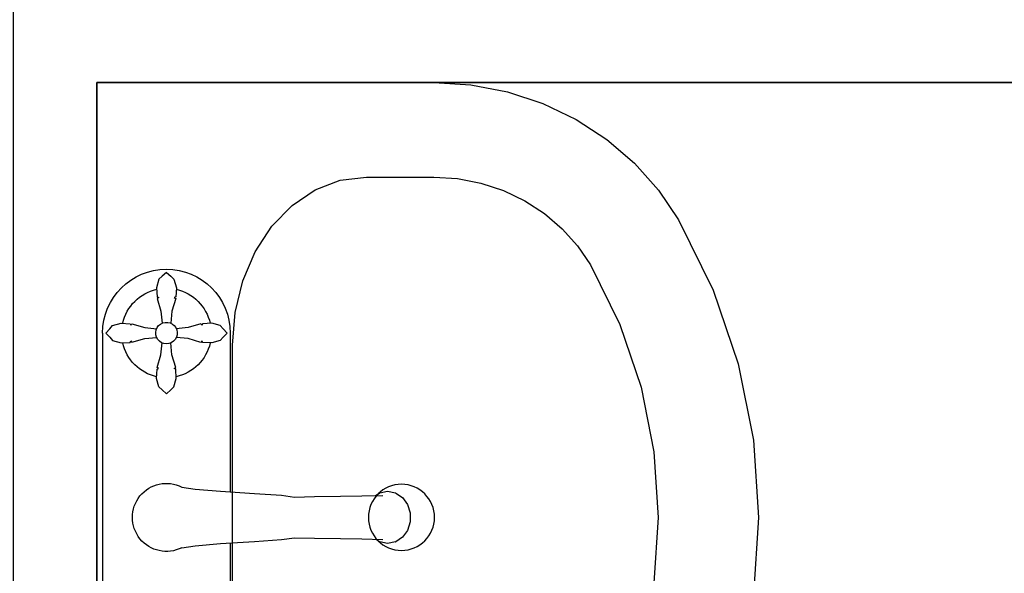
# Model space of a CAD drawing. Units: inches. Extents: x 3321 to 5237, y 11 to 1752.
# Tile 31 of 43: x 5059.68 to 5077.55, y 1416.43 to 1426.48. Entities that reach past the tile are written whole.
import ezdxf

# ---------------------------------------------------------------- set-up
doc = ezdxf.new("R2010")
doc.units = ezdxf.units.IN
for name, color, linetype, lineweight in [('A-ANNO-DIMS', 2, 'Continuous', 18), ('A-WALL', 7, 'Continuous', 35), ('Сантехника', 7, 'Continuous', 18)]:
    doc.layers.add(name, color=color, linetype=linetype, lineweight=lineweight)
doc.layers.add('SANTEH', color=7, linetype='Continuous')
doc.styles.get("Standard").update_dxf_attribs({"font": 'arial.ttf'})
doc.dimstyles.new('ISO-25', dxfattribs={"dimtxt": 9, "dimasz": 2.5, "dimexe": 1.25, "dimexo": 0.625, "dimtad": 1, "dimdec": 1, "dimlunit": 3, "dimtxsty": 'Standard', "dimcen": 2.5, "dimclrd": 4, "dimclre": 4, "dimclrt": 256, "dimadec": 0, "dimazin": 0, "dimtfac": 1, "dimtdec": 1, "dimtmove": 0, "dimatfit": 3, "dimfxl": 1, "dimarcsym": 0})

# ---------------------------------------------------------------- blocks, each defined once
blk = doc.blocks.new('Basin 01_71')
at = {"layer": 'SANTEH'}
for p, q in [((0.01, 350), (0.01, 171.82)), ((459.99, 350), (0.01, 350)), ((459.99, 350), (459.99, 171.82)), ((132.5, 345.3), (130.25, 343.2)), ((132.5, 345.3), (130.25, 343.2)), ((132.5, 345.3), (130.25, 343.2)), ((132.5, 345.3), (130.25, 343.2)), ((132.5, 345.3), (130.25, 343.2)), ((132.5, 345.3), (130.25, 343.2)), ((132.5, 346.95), (327.5, 346.95)), ((132.5, 345.3), (134.73, 343.2)), ((132.5, 345.3), (134.73, 343.2)), ((132.5, 345.3), (134.73, 343.2)), ((132.5, 345.3), (134.73, 343.2)), ((132.5, 345.3), (134.73, 343.2)), ((132.5, 345.3), (134.73, 343.2)), ((327.5, 345.3), (325.25, 343.2)), ((327.5, 345.3), (325.25, 343.2)), ((327.5, 345.3), (325.25, 343.2)), ((327.5, 345.3), (325.25, 343.2)), ((327.5, 345.3), (325.25, 343.2)), ((327.5, 345.3), (325.25, 343.2)), ((327.5, 345.3), (329.73, 343.2)), ((327.5, 345.3), (329.73, 343.2)), ((327.5, 345.3), (329.73, 343.2)), ((327.5, 345.3), (329.73, 343.2)), ((327.5, 345.3), (329.73, 343.2)), ((327.5, 345.3), (329.73, 343.2)), ((128.53, 341.7), (127.25, 337.2)), ((128.53, 341.7), (127.25, 337.2)), ((128.53, 341.7), (127.25, 337.2)), ((128.53, 341.7), (127.25, 337.2)), ((128.53, 341.7), (127.25, 337.2)), ((128.53, 341.7), (127.25, 337.2)), ((130.25, 343.2), (128.53, 341.7)), ((130.25, 343.2), (128.53, 341.7)), ((130.25, 343.2), (128.53, 341.7)), ((130.25, 343.2), (128.53, 341.7)), ((130.25, 343.2), (128.53, 341.7)), ((130.25, 343.2), (128.53, 341.7)), ((134.73, 343.2), (136.45, 341.7)), ((134.73, 343.2), (136.45, 341.7)), ((134.73, 343.2), (136.45, 341.7)), ((134.73, 343.2), (136.45, 341.7)), ((134.73, 343.2), (136.45, 341.7)), ((134.73, 343.2), (136.45, 341.7)), ((136.45, 341.7), (137.71, 337.2)), ((136.45, 341.7), (137.71, 337.2)), ((136.45, 341.7), (137.71, 337.2)), ((136.45, 341.7), (137.71, 337.2)), ((136.45, 341.7), (137.71, 337.2)), ((136.45, 341.7), (137.71, 337.2)), ((323.53, 341.7), (322.25, 337.2)), ((323.53, 341.7), (322.25, 337.2)), ((323.53, 341.7), (322.25, 337.2)), ((323.53, 341.7), (322.25, 337.2)), ((323.53, 341.7), (322.25, 337.2)), ((323.53, 341.7), (322.25, 337.2)), ((325.25, 343.2), (323.53, 341.7)), ((325.25, 343.2), (323.53, 341.7)), ((325.25, 343.2), (323.53, 341.7)), ((325.25, 343.2), (323.53, 341.7)), ((325.25, 343.2), (323.53, 341.7)), ((325.25, 343.2), (323.53, 341.7)), ((329.73, 343.2), (331.45, 341.7)), ((329.73, 343.2), (331.45, 341.7)), ((329.73, 343.2), (331.45, 341.7)), ((329.73, 343.2), (331.45, 341.7)), ((329.73, 343.2), (331.45, 341.7)), ((329.73, 343.2), (331.45, 341.7)), ((331.45, 341.7), (332.71, 337.2)), ((331.45, 341.7), (332.71, 337.2)), ((331.45, 341.7), (332.71, 337.2)), ((331.45, 341.7), (332.71, 337.2)), ((331.45, 341.7), (332.71, 337.2)), ((331.45, 341.7), (332.71, 337.2)), ((127.25, 337.2), (127.55, 332.32)), ((127.25, 337.2), (127.55, 332.32)), ((127.25, 337.2), (127.55, 332.32)), ((127.25, 337.2), (127.55, 332.32)), ((127.25, 337.2), (127.55, 332.32)), ((127.25, 337.2), (127.55, 332.32)), ((137.71, 337.2), (137.42, 332.32)), ((137.71, 337.2), (137.42, 332.32)), ((137.71, 337.2), (137.42, 332.32)), ((137.71, 337.2), (137.42, 332.32)), ((137.71, 337.2), (137.42, 332.32)), ((137.71, 337.2), (137.42, 332.32)), ((322.25, 337.2), (322.55, 332.32)), ((322.25, 337.2), (322.55, 332.32)), ((322.25, 337.2), (322.55, 332.32)), ((322.25, 337.2), (322.55, 332.32)), ((322.25, 337.2), (322.55, 332.32)), ((322.25, 337.2), (322.55, 332.32)), ((332.71, 337.2), (332.42, 332.32)), ((332.71, 337.2), (332.42, 332.32)), ((332.71, 337.2), (332.42, 332.32)), ((332.71, 337.2), (332.42, 332.32)), ((332.71, 337.2), (332.42, 332.32)), ((332.71, 337.2), (332.42, 332.32)), ((127.55, 332.32), (128.38, 332.02)), ((127.55, 332.32), (128.38, 332.02)), ((127.55, 332.32), (128.38, 332.02)), ((127.55, 332.32), (128.38, 332.02)), ((127.55, 332.32), (128.38, 332.02)), ((127.55, 332.32), (128.38, 332.02)), ((128.38, 332.02), (127.57, 331.46)), ((128.38, 332.02), (127.57, 331.46)), ((128.38, 332.02), (127.57, 331.46)), ((128.38, 332.02), (127.57, 331.46)), ((128.38, 332.02), (127.57, 331.46)), ((128.38, 332.02), (127.57, 331.46)), ((127.57, 331.46), (129.57, 324.71)), ((127.57, 331.46), (129.57, 324.71)), ((127.57, 331.46), (129.57, 324.71)), ((127.57, 331.46), (129.57, 324.71)), ((127.57, 331.46), (129.57, 324.71)), ((127.57, 331.46), (129.57, 324.71)), ((137.39, 331.46), (135.41, 324.71)), ((137.39, 331.46), (135.41, 324.71)), ((137.39, 331.46), (135.41, 324.71)), ((137.39, 331.46), (135.41, 324.71)), ((137.39, 331.46), (135.41, 324.71)), ((137.39, 331.46), (135.41, 324.71)), ((137.42, 332.32), (136.6, 332.02)), ((137.42, 332.32), (136.6, 332.02)), ((137.42, 332.32), (136.6, 332.02)), ((137.42, 332.32), (136.6, 332.02)), ((137.42, 332.32), (136.6, 332.02)), ((137.42, 332.32), (136.6, 332.02)), ((136.6, 332.02), (137.39, 331.46)), ((136.6, 332.02), (137.39, 331.46)), ((136.6, 332.02), (137.39, 331.46)), ((136.6, 332.02), (137.39, 331.46)), ((136.6, 332.02), (137.39, 331.46)), ((136.6, 332.02), (137.39, 331.46)), ((322.55, 332.32), (323.38, 332.02)), ((322.55, 332.32), (323.38, 332.02)), ((322.55, 332.32), (323.38, 332.02)), ((322.55, 332.32), (323.38, 332.02)), ((322.55, 332.32), (323.38, 332.02)), ((322.55, 332.32), (323.38, 332.02)), ((323.38, 332.02), (322.57, 331.46)), ((323.38, 332.02), (322.57, 331.46)), ((323.38, 332.02), (322.57, 331.46)), ((323.38, 332.02), (322.57, 331.46)), ((323.38, 332.02), (322.57, 331.46)), ((323.38, 332.02), (322.57, 331.46)), ((322.57, 331.46), (324.57, 324.71)), ((322.57, 331.46), (324.57, 324.71)), ((322.57, 331.46), (324.57, 324.71)), ((322.57, 331.46), (324.57, 324.71)), ((322.57, 331.46), (324.57, 324.71)), ((322.57, 331.46), (324.57, 324.71)), ((332.39, 331.46), (330.41, 324.71)), ((332.39, 331.46), (330.41, 324.71)), ((332.39, 331.46), (330.41, 324.71)), ((332.39, 331.46), (330.41, 324.71)), ((332.39, 331.46), (330.41, 324.71)), ((332.39, 331.46), (330.41, 324.71)), ((332.42, 332.32), (331.6, 332.02)), ((332.42, 332.32), (331.6, 332.02)), ((332.42, 332.32), (331.6, 332.02)), ((332.42, 332.32), (331.6, 332.02)), ((332.42, 332.32), (331.6, 332.02)), ((332.42, 332.32), (331.6, 332.02)), ((331.6, 332.02), (332.39, 331.46)), ((331.6, 332.02), (332.39, 331.46)), ((331.6, 332.02), (332.39, 331.46)), ((331.6, 332.02), (332.39, 331.46)), ((331.6, 332.02), (332.39, 331.46)), ((331.6, 332.02), (332.39, 331.46)), ((129.57, 324.71), (130.19, 318.36)), ((129.57, 324.71), (130.19, 318.36)), ((129.57, 324.71), (130.19, 318.36)), ((129.57, 324.71), (130.19, 318.36)), ((129.57, 324.71), (130.19, 318.36)), ((129.57, 324.71), (130.19, 318.36)), ((135.41, 324.71), (134.8, 318.4)), ((135.41, 324.71), (134.8, 318.4)), ((135.41, 324.71), (134.8, 318.4)), ((135.41, 324.71), (134.8, 318.4)), ((135.41, 324.71), (134.8, 318.4)), ((135.41, 324.71), (134.8, 318.4)), ((324.57, 324.71), (325.19, 318.36)), ((324.57, 324.71), (325.19, 318.36)), ((324.57, 324.71), (325.19, 318.36)), ((324.57, 324.71), (325.19, 318.36)), ((324.57, 324.71), (325.19, 318.36)), ((324.57, 324.71), (325.19, 318.36)), ((330.41, 324.71), (329.8, 318.4)), ((330.41, 324.71), (329.8, 318.4)), ((330.41, 324.71), (329.8, 318.4)), ((330.41, 324.71), (329.8, 318.4)), ((330.41, 324.71), (329.8, 318.4)), ((330.41, 324.71), (329.8, 318.4)), ((104, 317.15), (108.5, 318.41)), ((104, 317.15), (108.5, 318.41)), ((104, 317.15), (108.5, 318.41)), ((104, 317.15), (108.5, 318.41)), ((104, 317.15), (108.5, 318.41)), ((104, 317.15), (108.5, 318.41)), ((108.5, 318.41), (113.38, 318.11)), ((108.5, 318.41), (113.38, 318.11)), ((108.5, 318.41), (113.38, 318.11)), ((108.5, 318.41), (113.38, 318.11)), ((108.5, 318.41), (113.38, 318.11)), ((108.5, 318.41), (113.38, 318.11)), ((113.38, 318.11), (113.67, 317.29)), ((113.38, 318.11), (113.67, 317.29)), ((113.38, 318.11), (113.67, 317.29)), ((113.38, 318.11), (113.67, 317.29)), ((113.38, 318.11), (113.67, 317.29)), ((113.38, 318.11), (113.67, 317.29)), ((113.67, 317.29), (114.23, 318.09)), ((113.67, 317.29), (114.23, 318.09)), ((113.67, 317.29), (114.23, 318.09)), ((113.67, 317.29), (114.23, 318.09)), ((113.67, 317.29), (114.23, 318.09)), ((113.67, 317.29), (114.23, 318.09)), ((114.23, 318.09), (120.99, 316.1)), ((114.23, 318.09), (120.99, 316.1)), ((114.23, 318.09), (120.99, 316.1)), ((114.23, 318.09), (120.99, 316.1)), ((114.23, 318.09), (120.99, 316.1)), ((114.23, 318.09), (120.99, 316.1)), ((129.65, 318.13), (128.59, 317.34)), ((129.65, 318.13), (128.59, 317.34)), ((129.65, 318.13), (128.59, 317.34)), ((129.65, 318.13), (128.59, 317.34)), ((129.65, 318.13), (128.59, 317.34)), ((129.65, 318.13), (128.59, 317.34)), ((130.87, 318.66), (129.65, 318.13)), ((130.87, 318.66), (129.65, 318.13)), ((130.87, 318.66), (129.65, 318.13)), ((130.87, 318.66), (129.65, 318.13)), ((130.87, 318.66), (129.65, 318.13)), ((130.87, 318.66), (129.65, 318.13)), ((132.17, 318.89), (130.87, 318.66)), ((132.17, 318.89), (130.87, 318.66)), ((132.17, 318.89), (130.87, 318.66)), ((132.17, 318.89), (130.87, 318.66)), ((132.17, 318.89), (130.87, 318.66)), ((132.17, 318.89), (130.87, 318.66)), ((133.49, 318.81), (132.17, 318.89)), ((133.49, 318.81), (132.17, 318.89)), ((133.49, 318.81), (132.17, 318.89)), ((133.49, 318.81), (132.17, 318.89)), ((133.49, 318.81), (132.17, 318.89)), ((133.49, 318.81), (132.17, 318.89)), ((134.76, 318.43), (133.49, 318.81)), ((134.76, 318.43), (133.49, 318.81)), ((134.76, 318.43), (133.49, 318.81)), ((134.76, 318.43), (133.49, 318.81)), ((134.76, 318.43), (133.49, 318.81)), ((134.76, 318.43), (133.49, 318.81)), ((135.9, 317.77), (134.76, 318.43)), ((135.9, 317.77), (134.76, 318.43)), ((135.9, 317.77), (134.76, 318.43)), ((135.9, 317.77), (134.76, 318.43)), ((135.9, 317.77), (134.76, 318.43)), ((135.9, 317.77), (134.76, 318.43)), ((136.87, 316.86), (135.9, 317.77)), ((136.87, 316.86), (135.9, 317.77)), ((136.87, 316.86), (135.9, 317.77)), ((136.87, 316.86), (135.9, 317.77)), ((136.87, 316.86), (135.9, 317.77)), ((136.87, 316.86), (135.9, 317.77)), ((150.77, 318.12), (144.01, 316.12)), ((150.77, 318.12), (144.01, 316.12)), ((150.77, 318.12), (144.01, 316.12)), ((150.77, 318.12), (144.01, 316.12)), ((150.77, 318.12), (144.01, 316.12)), ((150.77, 318.12), (144.01, 316.12)), ((151.33, 317.32), (150.77, 318.12)), ((151.33, 317.32), (150.77, 318.12)), ((151.33, 317.32), (150.77, 318.12)), ((151.33, 317.32), (150.77, 318.12)), ((151.33, 317.32), (150.77, 318.12)), ((151.33, 317.32), (150.77, 318.12)), ((151.62, 318.15), (151.33, 317.32)), ((151.62, 318.15), (151.33, 317.32)), ((151.62, 318.15), (151.33, 317.32)), ((151.62, 318.15), (151.33, 317.32)), ((151.62, 318.15), (151.33, 317.32)), ((151.62, 318.15), (151.33, 317.32)), ((156.5, 318.45), (151.62, 318.15)), ((156.5, 318.45), (151.62, 318.15)), ((156.5, 318.45), (151.62, 318.15)), ((156.5, 318.45), (151.62, 318.15)), ((156.5, 318.45), (151.62, 318.15)), ((156.5, 318.45), (151.62, 318.15)), ((161, 317.17), (156.5, 318.45)), ((161, 317.17), (156.5, 318.45)), ((161, 317.17), (156.5, 318.45)), ((161, 317.17), (156.5, 318.45)), ((161, 317.17), (156.5, 318.45)), ((161, 317.17), (156.5, 318.45)), ((299, 317.15), (303.5, 318.41)), ((299, 317.15), (303.5, 318.41)), ((299, 317.15), (303.5, 318.41)), ((299, 317.15), (303.5, 318.41)), ((299, 317.15), (303.5, 318.41)), ((299, 317.15), (303.5, 318.41)), ((303.5, 318.41), (308.38, 318.11)), ((303.5, 318.41), (308.38, 318.11)), ((303.5, 318.41), (308.38, 318.11)), ((303.5, 318.41), (308.38, 318.11)), ((303.5, 318.41), (308.38, 318.11)), ((303.5, 318.41), (308.38, 318.11)), ((308.38, 318.11), (308.67, 317.29)), ((308.38, 318.11), (308.67, 317.29)), ((308.38, 318.11), (308.67, 317.29)), ((308.38, 318.11), (308.67, 317.29)), ((308.38, 318.11), (308.67, 317.29)), ((308.38, 318.11), (308.67, 317.29)), ((308.67, 317.29), (309.23, 318.09)), ((308.67, 317.29), (309.23, 318.09)), ((308.67, 317.29), (309.23, 318.09)), ((308.67, 317.29), (309.23, 318.09)), ((308.67, 317.29), (309.23, 318.09)), ((308.67, 317.29), (309.23, 318.09)), ((309.23, 318.09), (315.99, 316.1)), ((309.23, 318.09), (315.99, 316.1)), ((309.23, 318.09), (315.99, 316.1)), ((309.23, 318.09), (315.99, 316.1)), ((309.23, 318.09), (315.99, 316.1)), ((309.23, 318.09), (315.99, 316.1)), ((324.65, 318.13), (323.59, 317.34)), ((324.65, 318.13), (323.59, 317.34)), ((324.65, 318.13), (323.59, 317.34)), ((324.65, 318.13), (323.59, 317.34)), ((324.65, 318.13), (323.59, 317.34)), ((324.65, 318.13), (323.59, 317.34)), ((325.87, 318.66), (324.65, 318.13)), ((325.87, 318.66), (324.65, 318.13)), ((325.87, 318.66), (324.65, 318.13)), ((325.87, 318.66), (324.65, 318.13)), ((325.87, 318.66), (324.65, 318.13)), ((325.87, 318.66), (324.65, 318.13)), ((327.17, 318.89), (325.87, 318.66)), ((327.17, 318.89), (325.87, 318.66)), ((327.17, 318.89), (325.87, 318.66)), ((327.17, 318.89), (325.87, 318.66)), ((327.17, 318.89), (325.87, 318.66)), ((327.17, 318.89), (325.87, 318.66)), ((328.49, 318.81), (327.17, 318.89)), ((328.49, 318.81), (327.17, 318.89)), ((328.49, 318.81), (327.17, 318.89)), ((328.49, 318.81), (327.17, 318.89)), ((328.49, 318.81), (327.17, 318.89)), ((328.49, 318.81), (327.17, 318.89)), ((329.76, 318.43), (328.49, 318.81)), ((329.76, 318.43), (328.49, 318.81)), ((329.76, 318.43), (328.49, 318.81)), ((329.76, 318.43), (328.49, 318.81)), ((329.76, 318.43), (328.49, 318.81)), ((329.76, 318.43), (328.49, 318.81)), ((330.9, 317.77), (329.76, 318.43)), ((330.9, 317.77), (329.76, 318.43)), ((330.9, 317.77), (329.76, 318.43)), ((330.9, 317.77), (329.76, 318.43)), ((330.9, 317.77), (329.76, 318.43)), ((330.9, 317.77), (329.76, 318.43)), ((331.87, 316.86), (330.9, 317.77)), ((331.87, 316.86), (330.9, 317.77)), ((331.87, 316.86), (330.9, 317.77)), ((331.87, 316.86), (330.9, 317.77)), ((331.87, 316.86), (330.9, 317.77)), ((331.87, 316.86), (330.9, 317.77)), ((345.77, 318.12), (339.01, 316.12)), ((345.77, 318.12), (339.01, 316.12)), ((345.77, 318.12), (339.01, 316.12)), ((345.77, 318.12), (339.01, 316.12)), ((345.77, 318.12), (339.01, 316.12)), ((345.77, 318.12), (339.01, 316.12)), ((346.33, 317.32), (345.77, 318.12)), ((346.33, 317.32), (345.77, 318.12)), ((346.33, 317.32), (345.77, 318.12)), ((346.33, 317.32), (345.77, 318.12)), ((346.33, 317.32), (345.77, 318.12)), ((346.33, 317.32), (345.77, 318.12)), ((346.62, 318.15), (346.33, 317.32)), ((346.62, 318.15), (346.33, 317.32)), ((346.62, 318.15), (346.33, 317.32)), ((346.62, 318.15), (346.33, 317.32)), ((346.62, 318.15), (346.33, 317.32)), ((346.62, 318.15), (346.33, 317.32)), ((351.5, 318.45), (346.62, 318.15)), ((351.5, 318.45), (346.62, 318.15)), ((351.5, 318.45), (346.62, 318.15)), ((351.5, 318.45), (346.62, 318.15)), ((351.5, 318.45), (346.62, 318.15)), ((351.5, 318.45), (346.62, 318.15)), ((356, 317.17), (351.5, 318.45)), ((356, 317.17), (351.5, 318.45)), ((356, 317.17), (351.5, 318.45)), ((356, 317.17), (351.5, 318.45)), ((356, 317.17), (351.5, 318.45)), ((356, 317.17), (351.5, 318.45)), ((100.4, 313.2), (102.5, 315.43)), ((100.4, 313.2), (102.5, 315.43)), ((100.4, 313.2), (102.5, 315.43)), ((100.4, 313.2), (102.5, 315.43)), ((100.4, 313.2), (102.5, 315.43)), ((100.4, 313.2), (102.5, 315.43)), ((100.4, 313.2), (102.5, 310.95)), ((100.4, 313.2), (102.5, 310.95)), ((100.4, 313.2), (102.5, 310.95)), ((100.4, 313.2), (102.5, 310.95)), ((100.4, 313.2), (102.5, 310.95)), ((100.4, 313.2), (102.5, 310.95)), ((102.5, 315.43), (104, 317.15)), ((102.5, 315.43), (104, 317.15)), ((102.5, 315.43), (104, 317.15)), ((102.5, 315.43), (104, 317.15)), ((102.5, 315.43), (104, 317.15)), ((102.5, 315.43), (104, 317.15)), ((120.99, 316.1), (127.32, 315.5)), ((120.99, 316.1), (127.32, 315.5)), ((120.99, 316.1), (127.32, 315.5)), ((120.99, 316.1), (127.32, 315.5)), ((120.99, 316.1), (127.32, 315.5)), ((120.99, 316.1), (127.32, 315.5)), ((127.14, 315.15), (126.84, 313.86)), ((127.14, 315.15), (126.84, 313.86)), ((127.14, 315.15), (126.84, 313.86)), ((127.14, 315.15), (126.84, 313.86)), ((127.14, 315.15), (126.84, 313.86)), ((127.14, 315.15), (126.84, 313.86)), ((126.84, 313.86), (126.84, 312.54)), ((126.84, 313.86), (126.84, 312.54)), ((126.84, 313.86), (126.84, 312.54)), ((126.84, 313.86), (126.84, 312.54)), ((126.84, 313.86), (126.84, 312.54)), ((126.84, 313.86), (126.84, 312.54)), ((126.84, 312.54), (127.14, 311.25)), ((126.84, 312.54), (127.14, 311.25)), ((126.84, 312.54), (127.14, 311.25)), ((126.84, 312.54), (127.14, 311.25)), ((126.84, 312.54), (127.14, 311.25)), ((126.84, 312.54), (127.14, 311.25)), ((127.74, 316.33), (127.14, 315.15)), ((127.74, 316.33), (127.14, 315.15)), ((127.74, 316.33), (127.14, 315.15)), ((127.74, 316.33), (127.14, 315.15)), ((127.74, 316.33), (127.14, 315.15)), ((127.74, 316.33), (127.14, 315.15)), ((128.59, 317.34), (127.74, 316.33)), ((128.59, 317.34), (127.74, 316.33)), ((128.59, 317.34), (127.74, 316.33)), ((128.59, 317.34), (127.74, 316.33)), ((128.59, 317.34), (127.74, 316.33)), ((128.59, 317.34), (127.74, 316.33)), ((137.59, 315.76), (136.87, 316.86)), ((137.59, 315.76), (136.87, 316.86)), ((137.59, 315.76), (136.87, 316.86)), ((137.59, 315.76), (136.87, 316.86)), ((137.59, 315.76), (136.87, 316.86)), ((137.59, 315.76), (136.87, 316.86)), ((138.05, 314.51), (137.59, 315.76)), ((138.05, 314.51), (137.59, 315.76)), ((138.05, 314.51), (137.59, 315.76)), ((138.05, 314.51), (137.59, 315.76)), ((138.05, 314.51), (137.59, 315.76)), ((138.05, 314.51), (137.59, 315.76)), ((144.01, 316.12), (137.68, 315.51)), ((144.01, 316.12), (137.68, 315.51)), ((144.01, 316.12), (137.68, 315.51)), ((144.01, 316.12), (137.68, 315.51)), ((144.01, 316.12), (137.68, 315.51)), ((144.01, 316.12), (137.68, 315.51)), ((138.2, 313.2), (138.05, 314.51)), ((138.2, 313.2), (138.05, 314.51)), ((138.2, 313.2), (138.05, 314.51)), ((138.2, 313.2), (138.05, 314.51)), ((138.2, 313.2), (138.05, 314.51)), ((138.2, 313.2), (138.05, 314.51)), ((138.05, 311.88), (138.2, 313.2)), ((138.05, 311.88), (138.2, 313.2)), ((138.05, 311.88), (138.2, 313.2)), ((138.05, 311.88), (138.2, 313.2)), ((138.05, 311.88), (138.2, 313.2)), ((138.05, 311.88), (138.2, 313.2)), ((162.5, 315.45), (161, 317.17)), ((162.5, 315.45), (161, 317.17)), ((162.5, 315.45), (161, 317.17)), ((162.5, 315.45), (161, 317.17)), ((162.5, 315.45), (161, 317.17)), ((162.5, 315.45), (161, 317.17)), ((164.6, 313.2), (162.5, 315.45)), ((164.6, 313.2), (162.5, 315.45)), ((164.6, 313.2), (162.5, 315.45)), ((164.6, 313.2), (162.5, 315.45)), ((164.6, 313.2), (162.5, 315.45)), ((164.6, 313.2), (162.5, 315.45)), ((164.6, 313.2), (162.5, 310.96)), ((164.6, 313.2), (162.5, 310.96)), ((164.6, 313.2), (162.5, 310.96)), ((164.6, 313.2), (162.5, 310.96)), ((164.6, 313.2), (162.5, 310.96)), ((164.6, 313.2), (162.5, 310.96)), ((295.4, 313.2), (297.5, 315.43)), ((295.4, 313.2), (297.5, 315.43)), ((295.4, 313.2), (297.5, 315.43)), ((295.4, 313.2), (297.5, 315.43)), ((295.4, 313.2), (297.5, 315.43)), ((295.4, 313.2), (297.5, 315.43)), ((295.4, 313.2), (297.5, 310.95)), ((295.4, 313.2), (297.5, 310.95)), ((295.4, 313.2), (297.5, 310.95)), ((295.4, 313.2), (297.5, 310.95)), ((295.4, 313.2), (297.5, 310.95)), ((295.4, 313.2), (297.5, 310.95)), ((297.5, 315.43), (299, 317.15)), ((297.5, 315.43), (299, 317.15)), ((297.5, 315.43), (299, 317.15)), ((297.5, 315.43), (299, 317.15)), ((297.5, 315.43), (299, 317.15)), ((297.5, 315.43), (299, 317.15)), ((315.99, 316.1), (322.32, 315.5)), ((315.99, 316.1), (322.32, 315.5)), ((315.99, 316.1), (322.32, 315.5)), ((315.99, 316.1), (322.32, 315.5)), ((315.99, 316.1), (322.32, 315.5)), ((315.99, 316.1), (322.32, 315.5)), ((322.14, 315.15), (321.84, 313.86)), ((322.14, 315.15), (321.84, 313.86)), ((322.14, 315.15), (321.84, 313.86)), ((322.14, 315.15), (321.84, 313.86)), ((322.14, 315.15), (321.84, 313.86)), ((322.14, 315.15), (321.84, 313.86)), ((321.84, 313.86), (321.84, 312.54)), ((321.84, 313.86), (321.84, 312.54)), ((321.84, 313.86), (321.84, 312.54)), ((321.84, 313.86), (321.84, 312.54)), ((321.84, 313.86), (321.84, 312.54)), ((321.84, 313.86), (321.84, 312.54)), ((321.84, 312.54), (322.14, 311.25)), ((321.84, 312.54), (322.14, 311.25)), ((321.84, 312.54), (322.14, 311.25)), ((321.84, 312.54), (322.14, 311.25)), ((321.84, 312.54), (322.14, 311.25)), ((321.84, 312.54), (322.14, 311.25)), ((322.74, 316.33), (322.14, 315.15)), ((322.74, 316.33), (322.14, 315.15)), ((322.74, 316.33), (322.14, 315.15)), ((322.74, 316.33), (322.14, 315.15)), ((322.74, 316.33), (322.14, 315.15)), ((322.74, 316.33), (322.14, 315.15)), ((323.59, 317.34), (322.74, 316.33)), ((323.59, 317.34), (322.74, 316.33)), ((323.59, 317.34), (322.74, 316.33)), ((323.59, 317.34), (322.74, 316.33)), ((323.59, 317.34), (322.74, 316.33)), ((323.59, 317.34), (322.74, 316.33)), ((332.59, 315.76), (331.87, 316.86)), ((332.59, 315.76), (331.87, 316.86)), ((332.59, 315.76), (331.87, 316.86)), ((332.59, 315.76), (331.87, 316.86)), ((332.59, 315.76), (331.87, 316.86)), ((332.59, 315.76), (331.87, 316.86)), ((333.05, 314.51), (332.59, 315.76)), ((333.05, 314.51), (332.59, 315.76)), ((333.05, 314.51), (332.59, 315.76)), ((333.05, 314.51), (332.59, 315.76)), ((333.05, 314.51), (332.59, 315.76)), ((333.05, 314.51), (332.59, 315.76)), ((339.01, 316.12), (332.68, 315.51)), ((339.01, 316.12), (332.68, 315.51)), ((339.01, 316.12), (332.68, 315.51)), ((339.01, 316.12), (332.68, 315.51)), ((339.01, 316.12), (332.68, 315.51)), ((339.01, 316.12), (332.68, 315.51)), ((333.2, 313.2), (333.05, 314.51)), ((333.2, 313.2), (333.05, 314.51)), ((333.2, 313.2), (333.05, 314.51)), ((333.2, 313.2), (333.05, 314.51)), ((333.2, 313.2), (333.05, 314.51)), ((333.2, 313.2), (333.05, 314.51)), ((333.05, 311.88), (333.2, 313.2)), ((333.05, 311.88), (333.2, 313.2)), ((333.05, 311.88), (333.2, 313.2)), ((333.05, 311.88), (333.2, 313.2)), ((333.05, 311.88), (333.2, 313.2)), ((333.05, 311.88), (333.2, 313.2)), ((357.5, 315.45), (356, 317.17)), ((357.5, 315.45), (356, 317.17)), ((357.5, 315.45), (356, 317.17)), ((357.5, 315.45), (356, 317.17)), ((357.5, 315.45), (356, 317.17)), ((357.5, 315.45), (356, 317.17)), ((359.6, 313.2), (357.5, 315.45)), ((359.6, 313.2), (357.5, 315.45)), ((359.6, 313.2), (357.5, 315.45)), ((359.6, 313.2), (357.5, 315.45)), ((359.6, 313.2), (357.5, 315.45)), ((359.6, 313.2), (357.5, 315.45)), ((359.6, 313.2), (357.5, 310.96)), ((359.6, 313.2), (357.5, 310.96)), ((359.6, 313.2), (357.5, 310.96)), ((359.6, 313.2), (357.5, 310.96)), ((359.6, 313.2), (357.5, 310.96)), ((359.6, 313.2), (357.5, 310.96)), ((102.5, 310.95), (104, 309.22)), ((102.5, 310.95), (104, 309.22)), ((102.5, 310.95), (104, 309.22)), ((102.5, 310.95), (104, 309.22)), ((102.5, 310.95), (104, 309.22)), ((102.5, 310.95), (104, 309.22)), ((104, 309.22), (108.5, 307.95)), ((104, 309.22), (108.5, 307.95)), ((104, 309.22), (108.5, 307.95)), ((104, 309.22), (108.5, 307.95)), ((104, 309.22), (108.5, 307.95)), ((104, 309.22), (108.5, 307.95)), ((108.5, 307.95), (113.38, 308.25)), ((108.5, 307.95), (113.38, 308.25)), ((108.5, 307.95), (113.38, 308.25)), ((108.5, 307.95), (113.38, 308.25)), ((108.5, 307.95), (113.38, 308.25)), ((108.5, 307.95), (113.38, 308.25)), ((113.38, 308.25), (113.67, 309.07)), ((113.38, 308.25), (113.67, 309.07)), ((113.38, 308.25), (113.67, 309.07)), ((113.38, 308.25), (113.67, 309.07)), ((113.38, 308.25), (113.67, 309.07)), ((113.38, 308.25), (113.67, 309.07)), ((113.67, 309.07), (114.23, 308.27)), ((113.67, 309.07), (114.23, 308.27)), ((113.67, 309.07), (114.23, 308.27)), ((113.67, 309.07), (114.23, 308.27)), ((113.67, 309.07), (114.23, 308.27)), ((113.67, 309.07), (114.23, 308.27)), ((114.23, 308.27), (120.99, 310.27)), ((114.23, 308.27), (120.99, 310.27)), ((114.23, 308.27), (120.99, 310.27)), ((114.23, 308.27), (120.99, 310.27)), ((114.23, 308.27), (120.99, 310.27)), ((114.23, 308.27), (120.99, 310.27)), ((120.99, 310.27), (127.33, 310.88)), ((120.99, 310.27), (127.33, 310.88)), ((120.99, 310.27), (127.33, 310.88)), ((120.99, 310.27), (127.33, 310.88)), ((120.99, 310.27), (127.33, 310.88)), ((120.99, 310.27), (127.33, 310.88)), ((127.14, 311.25), (127.74, 310.06)), ((127.14, 311.25), (127.74, 310.06)), ((127.14, 311.25), (127.74, 310.06)), ((127.14, 311.25), (127.74, 310.06)), ((127.14, 311.25), (127.74, 310.06)), ((127.14, 311.25), (127.74, 310.06)), ((127.74, 310.06), (128.59, 309.05)), ((127.74, 310.06), (128.59, 309.05)), ((127.74, 310.06), (128.59, 309.05)), ((127.74, 310.06), (128.59, 309.05)), ((127.74, 310.06), (128.59, 309.05)), ((127.74, 310.06), (128.59, 309.05)), ((128.59, 309.05), (129.65, 308.26)), ((128.59, 309.05), (129.65, 308.26)), ((128.59, 309.05), (129.65, 308.26)), ((128.59, 309.05), (129.65, 308.26)), ((128.59, 309.05), (129.65, 308.26)), ((128.59, 309.05), (129.65, 308.26)), ((129.59, 301.68), (130.2, 308.02)), ((129.59, 301.68), (130.2, 308.02)), ((129.59, 301.68), (130.2, 308.02)), ((129.59, 301.68), (130.2, 308.02)), ((129.59, 301.68), (130.2, 308.02)), ((129.59, 301.68), (130.2, 308.02)), ((129.65, 308.26), (130.87, 307.74)), ((129.65, 308.26), (130.87, 307.74)), ((129.65, 308.26), (130.87, 307.74)), ((129.65, 308.26), (130.87, 307.74)), ((129.65, 308.26), (130.87, 307.74)), ((129.65, 308.26), (130.87, 307.74)), ((130.87, 307.74), (132.17, 307.51)), ((130.87, 307.74), (132.17, 307.51)), ((130.87, 307.74), (132.17, 307.51)), ((130.87, 307.74), (132.17, 307.51)), ((130.87, 307.74), (132.17, 307.51)), ((130.87, 307.74), (132.17, 307.51)), ((132.17, 307.51), (133.49, 307.58)), ((132.17, 307.51), (133.49, 307.58)), ((132.17, 307.51), (133.49, 307.58)), ((132.17, 307.51), (133.49, 307.58)), ((132.17, 307.51), (133.49, 307.58)), ((132.17, 307.51), (133.49, 307.58)), ((133.49, 307.58), (134.76, 307.96)), ((133.49, 307.58), (134.76, 307.96)), ((133.49, 307.58), (134.76, 307.96)), ((133.49, 307.58), (134.76, 307.96)), ((133.49, 307.58), (134.76, 307.96)), ((133.49, 307.58), (134.76, 307.96)), ((134.76, 307.96), (135.9, 308.62)), ((134.76, 307.96), (135.9, 308.62)), ((134.76, 307.96), (135.9, 308.62)), ((134.76, 307.96), (135.9, 308.62)), ((134.76, 307.96), (135.9, 308.62)), ((134.76, 307.96), (135.9, 308.62)), ((135.43, 301.68), (134.82, 308)), ((135.43, 301.68), (134.82, 308)), ((135.43, 301.68), (134.82, 308)), ((135.43, 301.68), (134.82, 308)), ((135.43, 301.68), (134.82, 308)), ((135.43, 301.68), (134.82, 308)), ((135.9, 308.62), (136.87, 309.53)), ((135.9, 308.62), (136.87, 309.53)), ((135.9, 308.62), (136.87, 309.53)), ((135.9, 308.62), (136.87, 309.53)), ((135.9, 308.62), (136.87, 309.53)), ((135.9, 308.62), (136.87, 309.53)), ((136.87, 309.53), (137.59, 310.64)), ((136.87, 309.53), (137.59, 310.64)), ((136.87, 309.53), (137.59, 310.64)), ((136.87, 309.53), (137.59, 310.64)), ((136.87, 309.53), (137.59, 310.64)), ((136.87, 309.53), (137.59, 310.64)), ((137.59, 310.64), (138.05, 311.88)), ((137.59, 310.64), (138.05, 311.88)), ((137.59, 310.64), (138.05, 311.88)), ((137.59, 310.64), (138.05, 311.88)), ((137.59, 310.64), (138.05, 311.88)), ((137.59, 310.64), (138.05, 311.88)), ((144.01, 310.29), (137.69, 310.9)), ((144.01, 310.29), (137.69, 310.9)), ((144.01, 310.29), (137.69, 310.9)), ((144.01, 310.29), (137.69, 310.9)), ((144.01, 310.29), (137.69, 310.9)), ((144.01, 310.29), (137.69, 310.9)), ((150.77, 308.3), (144.01, 310.29)), ((150.77, 308.3), (144.01, 310.29)), ((150.77, 308.3), (144.01, 310.29)), ((150.77, 308.3), (144.01, 310.29)), ((150.77, 308.3), (144.01, 310.29)), ((150.77, 308.3), (144.01, 310.29)), ((151.33, 309.1), (150.77, 308.3)), ((151.33, 309.1), (150.77, 308.3)), ((151.33, 309.1), (150.77, 308.3)), ((151.33, 309.1), (150.77, 308.3)), ((151.33, 309.1), (150.77, 308.3)), ((151.33, 309.1), (150.77, 308.3)), ((151.62, 308.28), (151.33, 309.1)), ((151.62, 308.28), (151.33, 309.1)), ((151.62, 308.28), (151.33, 309.1)), ((151.62, 308.28), (151.33, 309.1)), ((151.62, 308.28), (151.33, 309.1)), ((151.62, 308.28), (151.33, 309.1)), ((156.5, 307.98), (151.62, 308.28)), ((156.5, 307.98), (151.62, 308.28)), ((156.5, 307.98), (151.62, 308.28)), ((156.5, 307.98), (151.62, 308.28)), ((156.5, 307.98), (151.62, 308.28)), ((156.5, 307.98), (151.62, 308.28)), ((161, 309.25), (156.5, 307.98)), ((161, 309.25), (156.5, 307.98)), ((161, 309.25), (156.5, 307.98)), ((161, 309.25), (156.5, 307.98)), ((161, 309.25), (156.5, 307.98)), ((161, 309.25), (156.5, 307.98)), ((162.5, 310.96), (161, 309.25)), ((162.5, 310.96), (161, 309.25)), ((162.5, 310.96), (161, 309.25)), ((162.5, 310.96), (161, 309.25)), ((162.5, 310.96), (161, 309.25)), ((162.5, 310.96), (161, 309.25)), ((297.5, 310.95), (299, 309.22)), ((297.5, 310.95), (299, 309.22)), ((297.5, 310.95), (299, 309.22)), ((297.5, 310.95), (299, 309.22)), ((297.5, 310.95), (299, 309.22)), ((297.5, 310.95), (299, 309.22)), ((299, 309.22), (303.5, 307.95)), ((299, 309.22), (303.5, 307.95)), ((299, 309.22), (303.5, 307.95)), ((299, 309.22), (303.5, 307.95)), ((299, 309.22), (303.5, 307.95)), ((299, 309.22), (303.5, 307.95)), ((303.5, 307.95), (308.38, 308.25)), ((303.5, 307.95), (308.38, 308.25)), ((303.5, 307.95), (308.38, 308.25)), ((303.5, 307.95), (308.38, 308.25)), ((303.5, 307.95), (308.38, 308.25)), ((303.5, 307.95), (308.38, 308.25)), ((308.38, 308.25), (308.67, 309.07)), ((308.38, 308.25), (308.67, 309.07)), ((308.38, 308.25), (308.67, 309.07)), ((308.38, 308.25), (308.67, 309.07)), ((308.38, 308.25), (308.67, 309.07)), ((308.38, 308.25), (308.67, 309.07)), ((308.67, 309.07), (309.23, 308.27)), ((308.67, 309.07), (309.23, 308.27)), ((308.67, 309.07), (309.23, 308.27)), ((308.67, 309.07), (309.23, 308.27)), ((308.67, 309.07), (309.23, 308.27)), ((308.67, 309.07), (309.23, 308.27)), ((309.23, 308.27), (315.99, 310.27)), ((309.23, 308.27), (315.99, 310.27)), ((309.23, 308.27), (315.99, 310.27)), ((309.23, 308.27), (315.99, 310.27)), ((309.23, 308.27), (315.99, 310.27)), ((309.23, 308.27), (315.99, 310.27)), ((315.99, 310.27), (322.33, 310.88)), ((315.99, 310.27), (322.33, 310.88)), ((315.99, 310.27), (322.33, 310.88)), ((315.99, 310.27), (322.33, 310.88)), ((315.99, 310.27), (322.33, 310.88)), ((315.99, 310.27), (322.33, 310.88)), ((322.14, 311.25), (322.74, 310.06)), ((322.14, 311.25), (322.74, 310.06)), ((322.14, 311.25), (322.74, 310.06)), ((322.14, 311.25), (322.74, 310.06)), ((322.14, 311.25), (322.74, 310.06)), ((322.14, 311.25), (322.74, 310.06)), ((322.74, 310.06), (323.59, 309.05)), ((322.74, 310.06), (323.59, 309.05)), ((322.74, 310.06), (323.59, 309.05)), ((322.74, 310.06), (323.59, 309.05)), ((322.74, 310.06), (323.59, 309.05)), ((322.74, 310.06), (323.59, 309.05)), ((323.59, 309.05), (324.65, 308.26)), ((323.59, 309.05), (324.65, 308.26)), ((323.59, 309.05), (324.65, 308.26)), ((323.59, 309.05), (324.65, 308.26)), ((323.59, 309.05), (324.65, 308.26)), ((323.59, 309.05), (324.65, 308.26)), ((324.59, 301.68), (325.2, 308.02)), ((324.59, 301.68), (325.2, 308.02)), ((324.59, 301.68), (325.2, 308.02)), ((324.59, 301.68), (325.2, 308.02)), ((324.59, 301.68), (325.2, 308.02)), ((324.59, 301.68), (325.2, 308.02)), ((324.65, 308.26), (325.87, 307.74)), ((324.65, 308.26), (325.87, 307.74)), ((324.65, 308.26), (325.87, 307.74)), ((324.65, 308.26), (325.87, 307.74)), ((324.65, 308.26), (325.87, 307.74)), ((324.65, 308.26), (325.87, 307.74)), ((325.87, 307.74), (327.17, 307.51)), ((325.87, 307.74), (327.17, 307.51)), ((325.87, 307.74), (327.17, 307.51)), ((325.87, 307.74), (327.17, 307.51)), ((325.87, 307.74), (327.17, 307.51)), ((325.87, 307.74), (327.17, 307.51)), ((327.17, 307.51), (328.49, 307.58)), ((327.17, 307.51), (328.49, 307.58)), ((327.17, 307.51), (328.49, 307.58)), ((327.17, 307.51), (328.49, 307.58)), ((327.17, 307.51), (328.49, 307.58)), ((327.17, 307.51), (328.49, 307.58)), ((328.49, 307.58), (329.76, 307.96)), ((328.49, 307.58), (329.76, 307.96)), ((328.49, 307.58), (329.76, 307.96)), ((328.49, 307.58), (329.76, 307.96)), ((328.49, 307.58), (329.76, 307.96)), ((328.49, 307.58), (329.76, 307.96)), ((329.76, 307.96), (330.9, 308.62)), ((329.76, 307.96), (330.9, 308.62)), ((329.76, 307.96), (330.9, 308.62)), ((329.76, 307.96), (330.9, 308.62)), ((329.76, 307.96), (330.9, 308.62)), ((329.76, 307.96), (330.9, 308.62)), ((330.43, 301.68), (329.82, 308)), ((330.43, 301.68), (329.82, 308)), ((330.43, 301.68), (329.82, 308)), ((330.43, 301.68), (329.82, 308)), ((330.43, 301.68), (329.82, 308)), ((330.43, 301.68), (329.82, 308)), ((330.9, 308.62), (331.87, 309.53)), ((330.9, 308.62), (331.87, 309.53)), ((330.9, 308.62), (331.87, 309.53)), ((330.9, 308.62), (331.87, 309.53)), ((330.9, 308.62), (331.87, 309.53)), ((330.9, 308.62), (331.87, 309.53)), ((331.87, 309.53), (332.59, 310.64)), ((331.87, 309.53), (332.59, 310.64)), ((331.87, 309.53), (332.59, 310.64)), ((331.87, 309.53), (332.59, 310.64)), ((331.87, 309.53), (332.59, 310.64)), ((331.87, 309.53), (332.59, 310.64)), ((332.59, 310.64), (333.05, 311.88)), ((332.59, 310.64), (333.05, 311.88)), ((332.59, 310.64), (333.05, 311.88)), ((332.59, 310.64), (333.05, 311.88)), ((332.59, 310.64), (333.05, 311.88)), ((332.59, 310.64), (333.05, 311.88)), ((339.01, 310.29), (332.69, 310.9)), ((339.01, 310.29), (332.69, 310.9)), ((339.01, 310.29), (332.69, 310.9)), ((339.01, 310.29), (332.69, 310.9)), ((339.01, 310.29), (332.69, 310.9)), ((339.01, 310.29), (332.69, 310.9)), ((345.77, 308.3), (339.01, 310.29)), ((345.77, 308.3), (339.01, 310.29)), ((345.77, 308.3), (339.01, 310.29)), ((345.77, 308.3), (339.01, 310.29)), ((345.77, 308.3), (339.01, 310.29)), ((345.77, 308.3), (339.01, 310.29)), ((346.33, 309.1), (345.77, 308.3)), ((346.33, 309.1), (345.77, 308.3)), ((346.33, 309.1), (345.77, 308.3)), ((346.33, 309.1), (345.77, 308.3)), ((346.33, 309.1), (345.77, 308.3)), ((346.33, 309.1), (345.77, 308.3)), ((346.62, 308.28), (346.33, 309.1)), ((346.62, 308.28), (346.33, 309.1)), ((346.62, 308.28), (346.33, 309.1)), ((346.62, 308.28), (346.33, 309.1)), ((346.62, 308.28), (346.33, 309.1)), ((346.62, 308.28), (346.33, 309.1)), ((351.5, 307.98), (346.62, 308.28)), ((351.5, 307.98), (346.62, 308.28)), ((351.5, 307.98), (346.62, 308.28)), ((351.5, 307.98), (346.62, 308.28)), ((351.5, 307.98), (346.62, 308.28)), ((351.5, 307.98), (346.62, 308.28)), ((356, 309.25), (351.5, 307.98)), ((356, 309.25), (351.5, 307.98)), ((356, 309.25), (351.5, 307.98)), ((356, 309.25), (351.5, 307.98)), ((356, 309.25), (351.5, 307.98)), ((356, 309.25), (351.5, 307.98)), ((357.5, 310.96), (356, 309.25)), ((357.5, 310.96), (356, 309.25)), ((357.5, 310.96), (356, 309.25)), ((357.5, 310.96), (356, 309.25)), ((357.5, 310.96), (356, 309.25)), ((357.5, 310.96), (356, 309.25)), ((213.94, 305.07), (215, 298.02)), ((246.06, 305.07), (245, 298.02)), ((127.61, 294.93), (129.59, 301.68)), ((127.61, 294.93), (129.59, 301.68)), ((127.61, 294.93), (129.59, 301.68)), ((127.61, 294.93), (129.59, 301.68)), ((127.61, 294.93), (129.59, 301.68)), ((127.61, 294.93), (129.59, 301.68)), ((137.43, 294.93), (135.43, 301.68)), ((137.43, 294.93), (135.43, 301.68)), ((137.43, 294.93), (135.43, 301.68)), ((137.43, 294.93), (135.43, 301.68)), ((137.43, 294.93), (135.43, 301.68)), ((137.43, 294.93), (135.43, 301.68)), ((215, 298.02), (216.2, 284.6)), ((245, 298.02), (243.8, 284.6)), ((322.61, 294.93), (324.59, 301.68)), ((322.61, 294.93), (324.59, 301.68)), ((322.61, 294.93), (324.59, 301.68)), ((322.61, 294.93), (324.59, 301.68)), ((322.61, 294.93), (324.59, 301.68)), ((322.61, 294.93), (324.59, 301.68)), ((332.43, 294.93), (330.43, 301.68)), ((332.43, 294.93), (330.43, 301.68)), ((332.43, 294.93), (330.43, 301.68)), ((332.43, 294.93), (330.43, 301.68)), ((332.43, 294.93), (330.43, 301.68)), ((332.43, 294.93), (330.43, 301.68)), ((127.29, 289.2), (127.58, 294.07)), ((127.29, 289.2), (127.58, 294.07)), ((127.29, 289.2), (127.58, 294.07)), ((127.29, 289.2), (127.58, 294.07)), ((127.29, 289.2), (127.58, 294.07)), ((127.29, 289.2), (127.58, 294.07)), ((127.58, 294.07), (128.4, 294.37)), ((127.58, 294.07), (128.4, 294.37)), ((127.58, 294.07), (128.4, 294.37)), ((127.58, 294.07), (128.4, 294.37)), ((127.58, 294.07), (128.4, 294.37)), ((127.58, 294.07), (128.4, 294.37)), ((128.4, 294.37), (127.61, 294.93)), ((128.4, 294.37), (127.61, 294.93)), ((128.4, 294.37), (127.61, 294.93)), ((128.4, 294.37), (127.61, 294.93)), ((128.4, 294.37), (127.61, 294.93)), ((128.4, 294.37), (127.61, 294.93)), ((136.62, 294.37), (137.43, 294.93)), ((136.62, 294.37), (137.43, 294.93)), ((136.62, 294.37), (137.43, 294.93)), ((136.62, 294.37), (137.43, 294.93)), ((136.62, 294.37), (137.43, 294.93)), ((136.62, 294.37), (137.43, 294.93)), ((137.45, 294.07), (136.62, 294.37)), ((137.45, 294.07), (136.62, 294.37)), ((137.45, 294.07), (136.62, 294.37)), ((137.45, 294.07), (136.62, 294.37)), ((137.45, 294.07), (136.62, 294.37)), ((137.45, 294.07), (136.62, 294.37)), ((137.75, 289.2), (137.45, 294.07)), ((137.75, 289.2), (137.45, 294.07)), ((137.75, 289.2), (137.45, 294.07)), ((137.75, 289.2), (137.45, 294.07)), ((137.75, 289.2), (137.45, 294.07)), ((137.75, 289.2), (137.45, 294.07)), ((322.29, 289.2), (322.58, 294.07)), ((322.29, 289.2), (322.58, 294.07)), ((322.29, 289.2), (322.58, 294.07)), ((322.29, 289.2), (322.58, 294.07)), ((322.29, 289.2), (322.58, 294.07)), ((322.29, 289.2), (322.58, 294.07)), ((322.58, 294.07), (323.4, 294.37)), ((322.58, 294.07), (323.4, 294.37)), ((322.58, 294.07), (323.4, 294.37)), ((322.58, 294.07), (323.4, 294.37)), ((322.58, 294.07), (323.4, 294.37)), ((322.58, 294.07), (323.4, 294.37)), ((323.4, 294.37), (322.61, 294.93)), ((323.4, 294.37), (322.61, 294.93)), ((323.4, 294.37), (322.61, 294.93)), ((323.4, 294.37), (322.61, 294.93)), ((323.4, 294.37), (322.61, 294.93)), ((323.4, 294.37), (322.61, 294.93)), ((331.62, 294.37), (332.43, 294.93)), ((331.62, 294.37), (332.43, 294.93)), ((331.62, 294.37), (332.43, 294.93)), ((331.62, 294.37), (332.43, 294.93)), ((331.62, 294.37), (332.43, 294.93)), ((331.62, 294.37), (332.43, 294.93)), ((332.45, 294.07), (331.62, 294.37)), ((332.45, 294.07), (331.62, 294.37)), ((332.45, 294.07), (331.62, 294.37)), ((332.45, 294.07), (331.62, 294.37)), ((332.45, 294.07), (331.62, 294.37)), ((332.45, 294.07), (331.62, 294.37)), ((332.75, 289.2), (332.45, 294.07)), ((332.75, 289.2), (332.45, 294.07)), ((332.75, 289.2), (332.45, 294.07)), ((332.75, 289.2), (332.45, 294.07)), ((332.75, 289.2), (332.45, 294.07)), ((332.75, 289.2), (332.45, 294.07)), ((128.55, 284.7), (127.29, 289.2)), ((128.55, 284.7), (127.29, 289.2)), ((128.55, 284.7), (127.29, 289.2)), ((128.55, 284.7), (127.29, 289.2)), ((128.55, 284.7), (127.29, 289.2)), ((128.55, 284.7), (127.29, 289.2)), ((136.47, 284.7), (137.75, 289.2)), ((136.47, 284.7), (137.75, 289.2)), ((136.47, 284.7), (137.75, 289.2)), ((136.47, 284.7), (137.75, 289.2)), ((136.47, 284.7), (137.75, 289.2)), ((136.47, 284.7), (137.75, 289.2)), ((323.55, 284.7), (322.29, 289.2)), ((323.55, 284.7), (322.29, 289.2)), ((323.55, 284.7), (322.29, 289.2)), ((323.55, 284.7), (322.29, 289.2)), ((323.55, 284.7), (322.29, 289.2)), ((323.55, 284.7), (322.29, 289.2)), ((331.47, 284.7), (332.75, 289.2)), ((331.47, 284.7), (332.75, 289.2)), ((331.47, 284.7), (332.75, 289.2)), ((331.47, 284.7), (332.75, 289.2)), ((331.47, 284.7), (332.75, 289.2)), ((331.47, 284.7), (332.75, 289.2)), ((130.27, 283.2), (128.55, 284.7)), ((130.27, 283.2), (128.55, 284.7)), ((130.27, 283.2), (128.55, 284.7)), ((130.27, 283.2), (128.55, 284.7)), ((130.27, 283.2), (128.55, 284.7)), ((130.27, 283.2), (128.55, 284.7)), ((132.5, 281.1), (130.27, 283.2)), ((132.5, 281.1), (130.27, 283.2)), ((132.5, 281.1), (130.27, 283.2)), ((132.5, 281.1), (130.27, 283.2)), ((132.5, 281.1), (130.27, 283.2)), ((132.5, 281.1), (130.27, 283.2)), ((132.5, 281.1), (134.75, 283.2)), ((132.5, 281.1), (134.75, 283.2)), ((132.5, 281.1), (134.75, 283.2)), ((132.5, 281.1), (134.75, 283.2)), ((132.5, 281.1), (134.75, 283.2)), ((132.5, 281.1), (134.75, 283.2)), ((134.75, 283.2), (136.47, 284.7)), ((134.75, 283.2), (136.47, 284.7)), ((134.75, 283.2), (136.47, 284.7)), ((134.75, 283.2), (136.47, 284.7)), ((134.75, 283.2), (136.47, 284.7)), ((134.75, 283.2), (136.47, 284.7)), ((216.2, 284.6), (217.3, 266.64)), ((243.8, 284.6), (242.7, 266.64)), ((325.27, 283.2), (323.55, 284.7)), ((325.27, 283.2), (323.55, 284.7)), ((325.27, 283.2), (323.55, 284.7)), ((325.27, 283.2), (323.55, 284.7)), ((325.27, 283.2), (323.55, 284.7)), ((325.27, 283.2), (323.55, 284.7)), ((327.5, 281.1), (325.27, 283.2)), ((327.5, 281.1), (325.27, 283.2)), ((327.5, 281.1), (325.27, 283.2)), ((327.5, 281.1), (325.27, 283.2)), ((327.5, 281.1), (325.27, 283.2)), ((327.5, 281.1), (325.27, 283.2)), ((327.5, 281.1), (329.75, 283.2)), ((327.5, 281.1), (329.75, 283.2)), ((327.5, 281.1), (329.75, 283.2)), ((327.5, 281.1), (329.75, 283.2)), ((327.5, 281.1), (329.75, 283.2)), ((327.5, 281.1), (329.75, 283.2)), ((329.75, 283.2), (331.47, 284.7)), ((329.75, 283.2), (331.47, 284.7)), ((329.75, 283.2), (331.47, 284.7)), ((329.75, 283.2), (331.47, 284.7)), ((329.75, 283.2), (331.47, 284.7)), ((329.75, 283.2), (331.47, 284.7)), ((132.5, 279.45), (216.51, 279.45)), ((138.9, 278.22), (138.9, 278.2)), ((321.1, 278.2), (138.9, 278.2)), ((243.49, 279.45), (327.5, 279.45)), ((217.3, 266.64), (218.32, 252.37)), ((242.7, 266.64), (241.68, 252.37)), ((218.32, 252.37), (219.25, 245.4)), ((241.68, 252.37), (240.75, 245.4)), ((219.25, 245.4), (219.04, 234.84)), ((240.75, 245.4), (240.96, 234.84)), ((219.04, 234.84), (218.82, 221.06)), ((240.96, 234.84), (241.18, 221.06)), ((218.82, 221.06), (218.59, 209.77)), ((241.18, 221.06), (241.41, 209.77)), ((218.59, 209.77), (218.39, 198.72)), ((241.41, 209.77), (241.61, 198.72)), ((50, 207.45), (50, 171.82)), ((410, 207.45), (410, 171.82)), ((217.03, 200.28), (216.2, 196.2)), ((217.13, 200.56), (217.03, 200.28)), ((218.46, 202.55), (217.13, 200.56)), ((242.87, 200.56), (241.54, 202.55)), ((242.87, 200.56), (242.97, 200.28)), ((243.8, 196.2), (242.97, 200.28)), ((216.2, 196.2), (217.03, 192.11)), ((242.97, 192.11), (243.8, 196.2)), ((217.03, 192.11), (217.13, 191.83)), ((217.13, 191.83), (219.51, 188.27)), ((219.51, 188.27), (223.15, 185.62)), ((236.85, 185.62), (240.49, 188.27)), ((240.49, 188.27), (242.87, 191.83)), ((242.97, 192.11), (242.87, 191.83)), ((223.15, 185.62), (227.62, 184.21)), ((227.62, 184.21), (227.68, 184.21)), ((227.68, 184.21), (232.32, 184.21)), ((232.38, 184.21), (232.32, 184.21)), ((232.38, 184.21), (236.85, 185.62))]:
    blk.add_line(p, q, dxfattribs=at)
for points in [[(138.9, 278.22), (121.56, 276.86), (104.88, 272.84), (89.51, 266.3), (76.04, 257.5), (64.98, 246.77), (56.77, 234.54), (51.71, 221.26), (50, 207.45)], [(410, 207.45), (408.29, 221.26), (403.23, 234.54), (395.02, 246.77), (383.96, 257.5), (370.49, 266.3), (355.12, 272.84), (338.44, 276.86), (321.1, 278.22)], [(0, 171.82), (1.25, 152.11), (4.97, 132.75), (11.11, 114.09), (19.54, 96.48), (30.12, 80.22), (42.66, 65.6), (56.92, 52.9), (72.67, 42.34)], [(50, 171.82), (50.8, 159.2), (53.18, 146.81), (57.11, 134.88), (62.51, 123.6), (69.28, 113.2), (77.3, 103.84), (86.43, 95.71), (96.5, 88.96)], [(363.5, 88.96), (373.57, 95.71), (382.7, 103.84), (390.72, 113.2), (397.49, 123.6), (402.89, 134.88), (406.82, 146.81), (409.2, 159.2), (410, 171.82)], [(387.33, 42.34), (403.08, 52.9), (417.34, 65.6), (429.88, 80.22), (440.46, 96.48), (448.89, 114.09), (455.03, 132.75), (458.75, 152.11), (460, 171.82)], [(96.5, 88.96), (128.04, 73.42), (161.14, 62.15), (195.3, 55.32), (230, 53.03), (264.7, 55.32), (298.86, 62.15), (331.96, 73.42), (363.5, 88.96)], [(72.67, 42.34), (109.83, 24.03), (148.84, 10.75), (189.1, 2.7), (230, 0), (270.9, 2.7), (311.16, 10.75), (350.17, 24.03), (387.33, 42.34)]]:
    blk.add_lwpolyline(points, dxfattribs=at)
blk.add_circle((230, 188.89), 17.5, dxfattribs=at)
for centre, radius, start, end in [((132.5, 313.2), 33.75, 90, 270), ((327.5, 313.2), 33.75, 270, 90), ((132.5, 313.2), 23.7, 102.6646, 167.4213), ((132.5, 313.2), 23.7, 12.6646, 77.4213), ((327.5, 313.2), 23.7, 102.5787, 167.3354), ((327.5, 313.2), 23.7, 12.5787, 77.3354), ((230, 313.2), 18, 333.1469, 206.8531), ((132.5, 313.2), 23.7, 192.6646, 257.4213), ((132.5, 313.2), 23.7, 282.6646, 347.4213), ((327.5, 313.2), 23.7, 192.5787, 257.3354), ((327.5, 313.2), 23.7, 282.5787, 347.3354)]:
    blk.add_arc(centre, radius, start, end, dxfattribs=at)
blk = doc.blocks.new('*D199')
at = {"layer": 'A-ANNO-DIMS', "color": 4, "lineweight": -2, "transparency": 16777216}
for p, q in [((5059.569, 1379.636), (5059.569, 1473.411)), ((5060.444, 1379.636), (5058.319, 1379.636)), ((5059.569, 1372.136), (5059.569, 1377.136)), ((5060.444, 1369.636), (5058.319, 1369.636))]:
    blk.add_line(p, q, dxfattribs=at)
at = {"layer": 'A-ANNO-DIMS', "color": 4, "transparency": 16777216}
for points in [[(5059.153, 1377.136), (5059.986, 1377.136), (5059.569, 1379.636)], [(5059.153, 1372.136), (5059.986, 1372.136), (5059.569, 1369.636)]]:
    blk.add_solid(points, dxfattribs=at)
at = {"layer": 'Defpoints', "color": 0, "transparency": 16777216}
for p in [(5059.569, 1379.636), (5061.069, 1379.636), (5061.069, 1369.636)]:
    blk.add_point(p, dxfattribs=at)
at = {"layer": 'A-ANNO-DIMS', "transparency": 16777216, "insert": (5054.349, 1427.773), "char_height": 9, "attachment_point": 5, "rotation": 90}
blk.add_mtext('TAP 0\'-10" TYP.', dxfattribs=at)

msp = doc.modelspace()

# ---------------------------------------------------------------- linework, layer by layer
at = {"layer": 'A-WALL'}
for q in [(5061.084, 1341.339), (5087.084, 1425.339)]:
    msp.add_line((5061.084, 1425.339), q, dxfattribs=at)

# ---------------------------------------------------------------- block references
at = {"layer": 'Сантехника', "xscale": -0.0343047947041041, "yscale": 0.0343047947041041, "zscale": 0.0343047947041041, "rotation": 90}
msp.add_blockref('Basin 01_71', (5073.091, 1425.339), dxfattribs=at)

# ---------------------------------------------------------------- dimensions: what is measured, and where the dimension line sits
at = {"layer": 'A-ANNO-DIMS'}
dim = msp.add_linear_dim(base=(5059.569, 1379.636), p1=(5061.069, 1369.636), p2=(5061.069, 1379.636), angle=90, text='TAP <> TYP.', dimstyle='ISO-25', override={"dimdec": 1, "dimlfac": 1, "dimrnd": 0, "dimzin": 1, "dimdsep": 46, "dimlunit": 4, "dimfrac": 2}, dxfattribs=at)
dim.commit()
dim.dimension.update_dxf_attribs({"geometry": '*D199', "text_midpoint": (5054.349, 1427.773)})

doc.saveas('drawing.dxf')
